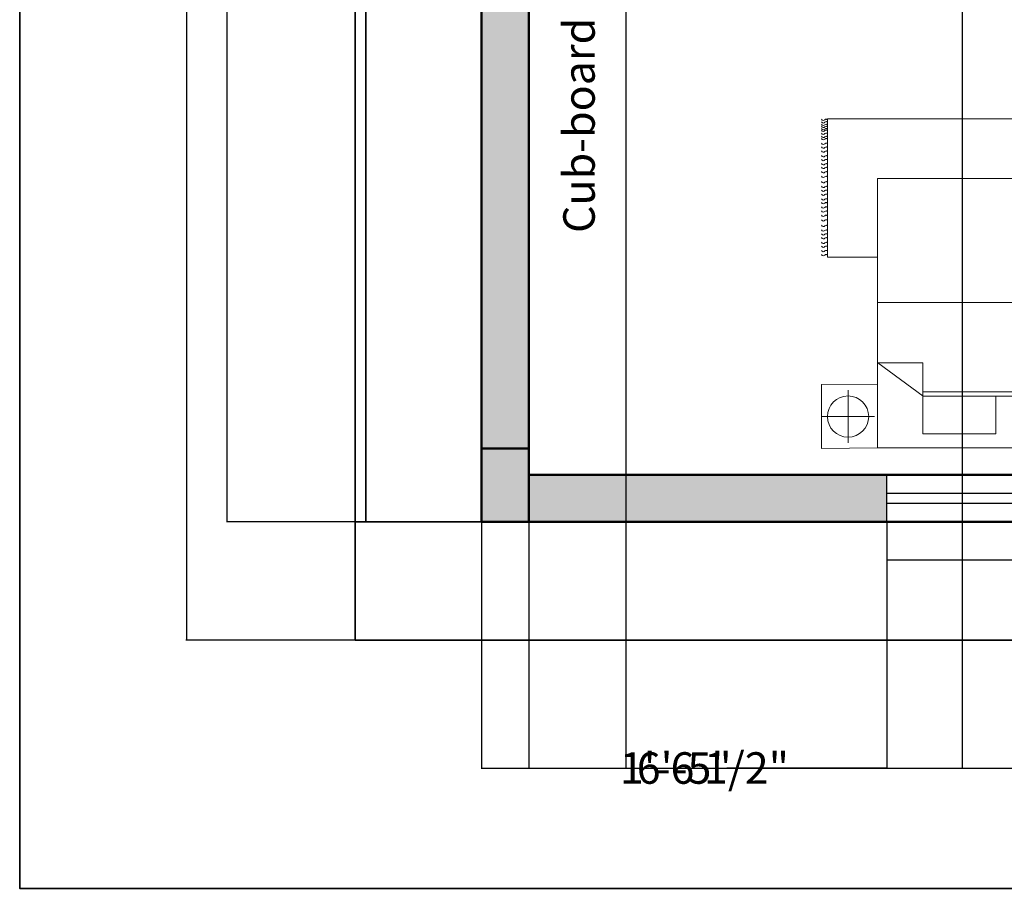
# Model space of a CAD drawing. Units: inches. Extents: x 1601 to 2080, y 5000 to 5589.
# Tile 1 of 11: x 1601 to 1788, y 5000 to 5165. Entities that reach past the tile are written whole.
import ezdxf

# ---------------------------------------------------------------- set-up
doc = ezdxf.new("R2010")
doc.units = ezdxf.units.IN
doc.header["$MEASUREMENT"] = 0
for name, color, linetype, lineweight in [('A-ANNO-DIMS', 2, 'Continuous', 18), ('A-ANNO-TEXT', 7, 'Continuous', 25), ('A-ANNO-TTLB', 7, 'Continuous', 35), ('A-COLS', 7, 'Continuous', 50), ('A-COLS-PATT', 18, 'Continuous', 13), ('A-FLOR-CASE', 8, 'Continuous', 25), ('A-FURN', 8, 'Continuous', 18), ('A-GLAZ', 4, 'Continuous', 25), ('A-WALL', 7, 'Continuous', 50), ('A-WALL-PATT', 241, 'Continuous', 13), ('C-PROP', 7, 'Continuous', 35)]:
    doc.layers.add(name, color=color, linetype=linetype, lineweight=lineweight)
doc.styles.get("Standard").update_dxf_attribs({"font": 'arial.ttf'})
doc.dimstyles.get("Standard").update_dxf_attribs({"dimtxt": 6, "dimasz": 0.18, "dimexe": 0.18, "dimexo": 0.0625, "dimgap": 0.09, "dimtad": 0, "dimtih": 1, "dimtoh": 1, "dimdec": 1, "dimzin": 0, "dimdsep": 46, "dimlunit": 3, "dimtxsty": 'Standard', "dimcen": 0.09, "dimadec": 0, "dimazin": 0, "dimtfac": 1, "dimtdec": 1, "dimtofl": 0, "dimtmove": 0, "dimatfit": 3, "dimfxl": 1, "dimtolj": 1, "dimtzin": 0, "dimarcsym": 0})

# ---------------------------------------------------------------- blocks, each defined once
blk = doc.blocks.new('*D4')
at = {"layer": 'A-ANNO-DIMS', "color": 0, "lineweight": -2, "transparency": 16777216}
for p, q in [((1664.35, 5509.2), (1632.18, 5509.2)), ((1632.36, 5509.02), (1632.36, 5281.35)), ((1632.36, 5047.39), (1632.36, 5275.05)), ((1664.35, 5047.21), (1632.18, 5047.21))]:
    blk.add_line(p, q, dxfattribs=at)
at = {"layer": 'A-ANNO-DIMS', "color": 0, "transparency": 16777216}
for points in [[(1632.33, 5509.02), (1632.39, 5509.02), (1632.36, 5509.2)], [(1632.33, 5047.39), (1632.39, 5047.39), (1632.36, 5047.21)]]:
    blk.add_solid(points, dxfattribs=at)
at = {"layer": 'Defpoints', "color": 0, "transparency": 16777216}
for p in [(1664.41, 5509.2), (1632.36, 5047.21), (1664.41, 5047.21)]:
    blk.add_point(p, dxfattribs=at)
at = {"layer": 'A-ANNO-DIMS', "color": 0, "transparency": 16777216, "insert": (1632.36, 5278.2), "char_height": 6, "attachment_point": 5}
blk.add_mtext("\\A1;40'", dxfattribs=at)
blk = doc.blocks.new('BED-DOUBLE-ENSEMBLE')
for p, q in [((5.6, 61.61), (5.6, 51.56)), ((63.65, 61.72), (63.65, 51.66)), ((10.63, 56.59), (0.57, 56.59)), ((68.68, 56.69), (58.62, 56.69)), ((49.39, 52.82), (10.63, 52.82)), ((49.39, 52.82), (58, 46.47)), ((49.44, 52.82), (49.44, 46.47)), ((49.44, 52), (10.63, 52)), ((49.44, 46.47), (58, 46.47)), ((58.05, 34.96), (10.63, 34.96)), ((4.35, 0), (4.35, 26.37)), ((4.35, 26.37), (10.65, 26.37)), ((58.05, 26.37), (67.59, 26.37)), ((67.59, 26.37), (67.59, 0)), ((67.59, 0), (4.35, 0))]:
    blk.add_line(p, q)
for points in [[(0, 50.39), (10.63, 50.5), (10.63, 62.68), (0, 62.58)], [(58.05, 62.68), (58.05, 11.36), (10.63, 11.36), (10.63, 62.68)], [(58.05, 50.5), (68.68, 50.6), (68.68, 62.78), (58.05, 62.68)], [(29.88, 59.98), (29.88, 52.82), (15.98, 52.82), (15.98, 59.98)], [(49.44, 59.98), (49.44, 52.82), (35.55, 52.82), (35.55, 59.98)]]:
    blk.add_lwpolyline(points, close=True)
for centre in [(5.6, 56.59), (63.65, 56.69)]:
    blk.add_circle(centre, 3.92)
for points, knots in [([(3.23, 25.83), (3.32, 25.96), (3.52, 26.2), (3.86, 25.96), (4.14, 25.78), (4.29, 25.89), (4.35, 25.94)], [0, 0, 0, 0, 0.400747, 0.791423, 1.067667, 1.29709, 1.29709, 1.29709, 1.29709]), ([(3.23, 25.06), (3.32, 25.18), (3.52, 25.42), (3.86, 25.18), (4.14, 25), (4.29, 25.11), (4.35, 25.16)], [0, 0, 0, 0, 0.400747, 0.791423, 1.067667, 1.29709, 1.29709, 1.29709, 1.29709]), ([(3.23, 24.24), (3.32, 24.36), (3.52, 24.6), (3.86, 24.36), (4.14, 24.19), (4.29, 24.3), (4.35, 24.34)], [0, 0, 0, 0, 0.400747, 0.791423, 1.067667, 1.29709, 1.29709, 1.29709, 1.29709]), ([(68.71, 25.83), (68.61, 25.96), (68.42, 26.2), (68.08, 25.96), (67.8, 25.78), (67.65, 25.89), (67.58, 25.94)], [0, 0, 0, 0, 0.400747, 0.791423, 1.067667, 1.29709, 1.29709, 1.29709, 1.29709]), ([(68.71, 25.06), (68.61, 25.18), (68.42, 25.42), (68.08, 25.18), (67.8, 25), (67.65, 25.11), (67.58, 25.16)], [0, 0, 0, 0, 0.400747, 0.791423, 1.067667, 1.29709, 1.29709, 1.29709, 1.29709]), ([(68.71, 24.24), (68.61, 24.36), (68.42, 24.6), (68.08, 24.36), (67.8, 24.19), (67.65, 24.3), (67.58, 24.34)], [0, 0, 0, 0, 0.400747, 0.791423, 1.067667, 1.29709, 1.29709, 1.29709, 1.29709]), ([(3.23, 23.51), (3.32, 23.63), (3.52, 23.87), (3.86, 23.63), (4.14, 23.46), (4.29, 23.57), (4.35, 23.62)], [0, 0, 0, 0, 0.400747, 0.791423, 1.067667, 1.29709, 1.29709, 1.29709, 1.29709]), ([(3.23, 22.63), (3.32, 22.75), (3.52, 22.99), (3.86, 22.75), (4.14, 22.58), (4.29, 22.68), (4.35, 22.73)], [0, 0, 0, 0, 0.400747, 0.791423, 1.067667, 1.29709, 1.29709, 1.29709, 1.29709]), ([(68.71, 23.51), (68.61, 23.63), (68.42, 23.87), (68.08, 23.63), (67.8, 23.46), (67.65, 23.57), (67.58, 23.62)], [0, 0, 0, 0, 0.400747, 0.791423, 1.067667, 1.29709, 1.29709, 1.29709, 1.29709]), ([(68.71, 22.63), (68.61, 22.75), (68.42, 22.99), (68.08, 22.75), (67.8, 22.58), (67.65, 22.68), (67.58, 22.73)], [0, 0, 0, 0, 0.400747, 0.791423, 1.067667, 1.29709, 1.29709, 1.29709, 1.29709]), ([(3.23, 21.88), (3.32, 22), (3.52, 22.24), (3.86, 22), (4.14, 21.83), (4.29, 21.93), (4.35, 21.98)], [0, 0, 0, 0, 0.400747, 0.791423, 1.067667, 1.29709, 1.29709, 1.29709, 1.29709]), ([(3.23, 21.15), (3.32, 21.27), (3.52, 21.51), (3.86, 21.27), (4.14, 21.1), (4.29, 21.2), (4.35, 21.25)], [0, 0, 0, 0, 0.400747, 0.791423, 1.067667, 1.29709, 1.29709, 1.29709, 1.29709]), ([(68.71, 21.88), (68.61, 22), (68.42, 22.24), (68.08, 22), (67.8, 21.83), (67.65, 21.93), (67.58, 21.98)], [0, 0, 0, 0, 0.400747, 0.791423, 1.067667, 1.29709, 1.29709, 1.29709, 1.29709]), ([(68.71, 21.15), (68.61, 21.27), (68.42, 21.51), (68.08, 21.27), (67.8, 21.1), (67.65, 21.2), (67.58, 21.25)], [0, 0, 0, 0, 0.400747, 0.791423, 1.067667, 1.29709, 1.29709, 1.29709, 1.29709]), ([(3.23, 20.27), (3.32, 20.39), (3.52, 20.63), (3.86, 20.39), (4.14, 20.22), (4.29, 20.32), (4.35, 20.37)], [0, 0, 0, 0, 0.400747, 0.791423, 1.067667, 1.29709, 1.29709, 1.29709, 1.29709]), ([(3.23, 19.23), (3.32, 19.35), (3.52, 19.59), (3.86, 19.35), (4.14, 19.18), (4.29, 19.29), (4.35, 19.33)], [0, 0, 0, 0, 0.400747, 0.791423, 1.067667, 1.29709, 1.29709, 1.29709, 1.29709]), ([(68.71, 20.27), (68.61, 20.39), (68.42, 20.63), (68.08, 20.39), (67.8, 20.22), (67.65, 20.32), (67.58, 20.37)], [0, 0, 0, 0, 0.400747, 0.791423, 1.067667, 1.29709, 1.29709, 1.29709, 1.29709]), ([(68.71, 19.23), (68.61, 19.35), (68.42, 19.59), (68.08, 19.35), (67.8, 19.18), (67.65, 19.29), (67.58, 19.33)], [0, 0, 0, 0, 0.400747, 0.791423, 1.067667, 1.29709, 1.29709, 1.29709, 1.29709]), ([(3.23, 18.35), (3.32, 18.47), (3.52, 18.71), (3.86, 18.47), (4.14, 18.3), (4.29, 18.4), (4.35, 18.45)], [0, 0, 0, 0, 0.400747, 0.791423, 1.067667, 1.29709, 1.29709, 1.29709, 1.29709]), ([(3.23, 17.53), (3.32, 17.65), (3.52, 17.89), (3.86, 17.65), (4.14, 17.48), (4.29, 17.59), (4.35, 17.64)], [0, 0, 0, 0, 0.400747, 0.791423, 1.067667, 1.29709, 1.29709, 1.29709, 1.29709]), ([(3.23, 16.76), (3.32, 16.88), (3.52, 17.12), (3.86, 16.88), (4.14, 16.7), (4.29, 16.81), (4.35, 16.86)], [0, 0, 0, 0, 0.400747, 0.791423, 1.067667, 1.29709, 1.29709, 1.29709, 1.29709]), ([(68.71, 18.35), (68.61, 18.47), (68.42, 18.71), (68.08, 18.47), (67.8, 18.3), (67.65, 18.4), (67.58, 18.45)], [0, 0, 0, 0, 0.400747, 0.791423, 1.067667, 1.29709, 1.29709, 1.29709, 1.29709]), ([(68.71, 17.53), (68.61, 17.65), (68.42, 17.89), (68.08, 17.65), (67.8, 17.48), (67.65, 17.59), (67.58, 17.64)], [0, 0, 0, 0, 0.400747, 0.791423, 1.067667, 1.29709, 1.29709, 1.29709, 1.29709]), ([(68.71, 16.76), (68.61, 16.88), (68.42, 17.12), (68.08, 16.88), (67.8, 16.7), (67.65, 16.81), (67.58, 16.86)], [0, 0, 0, 0, 0.400747, 0.791423, 1.067667, 1.29709, 1.29709, 1.29709, 1.29709]), ([(3.23, 15.94), (3.32, 16.06), (3.52, 16.3), (3.86, 16.06), (4.14, 15.89), (4.29, 15.99), (4.35, 16.04)], [0, 0, 0, 0, 0.400747, 0.791423, 1.067667, 1.29709, 1.29709, 1.29709, 1.29709]), ([(3.23, 15.21), (3.32, 15.33), (3.52, 15.57), (3.86, 15.33), (4.14, 15.16), (4.29, 15.27), (4.35, 15.31)], [0, 0, 0, 0, 0.400747, 0.791423, 1.067667, 1.29709, 1.29709, 1.29709, 1.29709]), ([(68.71, 15.94), (68.61, 16.06), (68.42, 16.3), (68.08, 16.06), (67.8, 15.89), (67.65, 15.99), (67.58, 16.04)], [0, 0, 0, 0, 0.400747, 0.791423, 1.067667, 1.29709, 1.29709, 1.29709, 1.29709]), ([(68.71, 15.21), (68.61, 15.33), (68.42, 15.57), (68.08, 15.33), (67.8, 15.16), (67.65, 15.27), (67.58, 15.31)], [0, 0, 0, 0, 0.400747, 0.791423, 1.067667, 1.29709, 1.29709, 1.29709, 1.29709]), ([(3.23, 14.33), (3.32, 14.45), (3.52, 14.69), (3.86, 14.45), (4.14, 14.28), (4.29, 14.38), (4.35, 14.43)], [0, 0, 0, 0, 0.400747, 0.791423, 1.067667, 1.29709, 1.29709, 1.29709, 1.29709]), ([(3.23, 13.58), (3.32, 13.7), (3.52, 13.94), (3.86, 13.7), (4.14, 13.53), (4.29, 13.63), (4.35, 13.68)], [0, 0, 0, 0, 0.400747, 0.791423, 1.067667, 1.29709, 1.29709, 1.29709, 1.29709]), ([(3.23, 12.85), (3.32, 12.97), (3.52, 13.21), (3.86, 12.97), (4.14, 12.8), (4.29, 12.9), (4.35, 12.95)], [0, 0, 0, 0, 0.400747, 0.791423, 1.067667, 1.29709, 1.29709, 1.29709, 1.29709]), ([(68.71, 14.33), (68.61, 14.45), (68.42, 14.69), (68.08, 14.45), (67.8, 14.28), (67.65, 14.38), (67.58, 14.43)], [0, 0, 0, 0, 0.400747, 0.791423, 1.067667, 1.29709, 1.29709, 1.29709, 1.29709]), ([(68.71, 13.58), (68.61, 13.7), (68.42, 13.94), (68.08, 13.7), (67.8, 13.53), (67.65, 13.63), (67.58, 13.68)], [0, 0, 0, 0, 0.400747, 0.791423, 1.067667, 1.29709, 1.29709, 1.29709, 1.29709]), ([(68.71, 12.85), (68.61, 12.97), (68.42, 13.21), (68.08, 12.97), (67.8, 12.8), (67.65, 12.9), (67.58, 12.95)], [0, 0, 0, 0, 0.400747, 0.791423, 1.067667, 1.29709, 1.29709, 1.29709, 1.29709]), ([(3.23, 11.97), (3.32, 12.09), (3.52, 12.33), (3.86, 12.09), (4.14, 11.92), (4.29, 12.02), (4.35, 12.07)], [0, 0, 0, 0, 0.400747, 0.791423, 1.067667, 1.29709, 1.29709, 1.29709, 1.29709]), ([(68.71, 11.97), (68.61, 12.09), (68.42, 12.33), (68.08, 12.09), (67.8, 11.92), (67.65, 12.02), (67.58, 12.07)], [0, 0, 0, 0, 0.400747, 0.791423, 1.067667, 1.29709, 1.29709, 1.29709, 1.29709]), ([(3.23, 10.93), (3.32, 11.05), (3.52, 11.29), (3.86, 11.05), (4.14, 10.88), (4.29, 10.99), (4.35, 11.03)], [0, 0, 0, 0, 0.400747, 0.791423, 1.067667, 1.29709, 1.29709, 1.29709, 1.29709]), ([(3.23, 10.05), (3.32, 10.17), (3.52, 10.41), (3.86, 10.17), (4.14, 10), (4.29, 10.1), (4.35, 10.15)], [0, 0, 0, 0, 0.400747, 0.791423, 1.067667, 1.29709, 1.29709, 1.29709, 1.29709]), ([(3.23, 9.23), (3.32, 9.35), (3.52, 9.59), (3.86, 9.35), (4.14, 9.18), (4.29, 9.29), (4.35, 9.34)], [0, 0, 0, 0, 0.400747, 0.791423, 1.067667, 1.29709, 1.29709, 1.29709, 1.29709]), ([(68.71, 10.93), (68.61, 11.05), (68.42, 11.29), (68.08, 11.05), (67.8, 10.88), (67.65, 10.99), (67.58, 11.03)], [0, 0, 0, 0, 0.400747, 0.791423, 1.067667, 1.29709, 1.29709, 1.29709, 1.29709]), ([(68.71, 10.05), (68.61, 10.17), (68.42, 10.41), (68.08, 10.17), (67.8, 10), (67.65, 10.1), (67.58, 10.15)], [0, 0, 0, 0, 0.400747, 0.791423, 1.067667, 1.29709, 1.29709, 1.29709, 1.29709]), ([(68.71, 9.23), (68.61, 9.35), (68.42, 9.59), (68.08, 9.35), (67.8, 9.18), (67.65, 9.29), (67.58, 9.34)], [0, 0, 0, 0, 0.400747, 0.791423, 1.067667, 1.29709, 1.29709, 1.29709, 1.29709]), ([(3.23, 8.54), (3.32, 8.66), (3.52, 8.9), (3.86, 8.66), (4.14, 8.49), (4.29, 8.6), (4.35, 8.65)], [0, 0, 0, 0, 0.400747, 0.791423, 1.067667, 1.29709, 1.29709, 1.29709, 1.29709]), ([(3.23, 7.73), (3.32, 7.85), (3.52, 8.09), (3.86, 7.85), (4.14, 7.67), (4.29, 7.78), (4.35, 7.83)], [0, 0, 0, 0, 0.400747, 0.791423, 1.067667, 1.29709, 1.29709, 1.29709, 1.29709]), ([(68.71, 8.54), (68.61, 8.66), (68.42, 8.9), (68.08, 8.66), (67.8, 8.49), (67.65, 8.6), (67.58, 8.65)], [0, 0, 0, 0, 0.400747, 0.791423, 1.067667, 1.29709, 1.29709, 1.29709, 1.29709]), ([(68.71, 7.73), (68.61, 7.85), (68.42, 8.09), (68.08, 7.85), (67.8, 7.67), (67.65, 7.78), (67.58, 7.83)], [0, 0, 0, 0, 0.400747, 0.791423, 1.067667, 1.29709, 1.29709, 1.29709, 1.29709]), ([(3.23, 7), (3.32, 7.12), (3.52, 7.36), (3.86, 7.12), (4.14, 6.95), (4.29, 7.05), (4.35, 7.1)], [0, 0, 0, 0, 0.400747, 0.791423, 1.067667, 1.29709, 1.29709, 1.29709, 1.29709]), ([(3.23, 6.12), (3.32, 6.24), (3.52, 6.48), (3.86, 6.24), (4.14, 6.06), (4.29, 6.17), (4.35, 6.22)], [0, 0, 0, 0, 0.400747, 0.791423, 1.067667, 1.29709, 1.29709, 1.29709, 1.29709]), ([(3.23, 5.36), (3.32, 5.49), (3.52, 5.72), (3.86, 5.49), (4.14, 5.31), (4.29, 5.42), (4.35, 5.47)], [0, 0, 0, 0, 0.400747, 0.791423, 1.067667, 1.29709, 1.29709, 1.29709, 1.29709]), ([(68.71, 7), (68.61, 7.12), (68.42, 7.36), (68.08, 7.12), (67.8, 6.95), (67.65, 7.05), (67.58, 7.1)], [0, 0, 0, 0, 0.400747, 0.791423, 1.067667, 1.29709, 1.29709, 1.29709, 1.29709]), ([(68.71, 6.12), (68.61, 6.24), (68.42, 6.48), (68.08, 6.24), (67.8, 6.06), (67.65, 6.17), (67.58, 6.22)], [0, 0, 0, 0, 0.400747, 0.791423, 1.067667, 1.29709, 1.29709, 1.29709, 1.29709]), ([(68.71, 5.36), (68.61, 5.49), (68.42, 5.72), (68.08, 5.49), (67.8, 5.31), (67.65, 5.42), (67.58, 5.47)], [0, 0, 0, 0, 0.400747, 0.791423, 1.067667, 1.29709, 1.29709, 1.29709, 1.29709]), ([(3.23, 4.64), (3.32, 4.76), (3.52, 5), (3.86, 4.76), (4.14, 4.58), (4.29, 4.69), (4.35, 4.74)], [0, 0, 0, 0, 0.400747, 0.791423, 1.067667, 1.29709, 1.29709, 1.29709, 1.29709]), ([(3.23, 3.75), (3.32, 3.88), (3.52, 4.11), (3.86, 3.88), (4.14, 3.7), (4.29, 3.81), (4.35, 3.86)], [0, 0, 0, 0, 0.400747, 0.791423, 1.067667, 1.29709, 1.29709, 1.29709, 1.29709]), ([(68.71, 4.64), (68.61, 4.76), (68.42, 5), (68.08, 4.76), (67.8, 4.59), (67.66, 4.69), (67.59, 4.73)], [0, 0, 0, 0, 0.400747, 0.791423, 1.067667, 1.283686, 1.283686, 1.283686, 1.283686]), ([(68.71, 3.75), (68.61, 3.88), (68.42, 4.11), (68.08, 3.88), (67.8, 3.7), (67.66, 3.8), (67.59, 3.85)], [0, 0, 0, 0, 0.400747, 0.791423, 1.067667, 1.283686, 1.283686, 1.283686, 1.283686]), ([(3.23, 3.32), (3.32, 3.45), (3.51, 3.7), (3.86, 3.44), (4.14, 3.27), (4.29, 3.38), (4.35, 3.43)], [0, 0, 0, 0, 0.407265, 0.802015, 1.07826, 1.307683, 1.307683, 1.307683, 1.307683]), ([(3.23, 2.76), (3.32, 2.88), (3.52, 3.12), (3.86, 2.88), (4.14, 2.71), (4.29, 2.81), (4.35, 2.86)], [0, 0, 0, 0, 0.400747, 0.791423, 1.067667, 1.29709, 1.29709, 1.29709, 1.29709]), ([(3.23, 2.18), (3.32, 2.31), (3.52, 2.54), (3.86, 2.31), (4.14, 2.13), (4.29, 2.24), (4.35, 2.29)], [0, 0, 0, 0, 0.400747, 0.791423, 1.067667, 1.29709, 1.29709, 1.29709, 1.29709]), ([(3.23, 1.88), (3.32, 2), (3.52, 2.24), (3.86, 2), (4.14, 1.82), (4.29, 1.93), (4.35, 1.98)], [0, 0, 0, 0, 0.400747, 0.791423, 1.067667, 1.29709, 1.29709, 1.29709, 1.29709]), ([(68.71, 3.32), (68.61, 3.45), (68.42, 3.69), (68.08, 3.45), (67.8, 3.27), (67.66, 3.38), (67.59, 3.42)], [0, 0, 0, 0, 0.402903, 0.794912, 1.071156, 1.287177, 1.287177, 1.287177, 1.287177]), ([(68.71, 2.73), (68.61, 2.85), (68.42, 3.09), (68.08, 2.85), (67.8, 2.68), (67.66, 2.78), (67.59, 2.82)], [0, 0, 0, 0, 0.400747, 0.791423, 1.067667, 1.283686, 1.283686, 1.283686, 1.283686]), ([(68.71, 2.16), (68.61, 2.28), (68.42, 2.52), (68.08, 2.28), (67.8, 2.11), (67.66, 2.21), (67.59, 2.25)], [0, 0, 0, 0, 0.400747, 0.791423, 1.067667, 1.283686, 1.283686, 1.283686, 1.283686]), ([(68.71, 1.85), (68.61, 1.97), (68.42, 2.21), (68.08, 1.97), (67.8, 1.8), (67.66, 1.9), (67.59, 1.94)], [0, 0, 0, 0, 0.400747, 0.791423, 1.067667, 1.283686, 1.283686, 1.283686, 1.283686]), ([(3.23, 1.46), (3.32, 1.58), (3.52, 1.82), (3.86, 1.58), (4.14, 1.4), (4.29, 1.51), (4.35, 1.56)], [0, 0, 0, 0, 0.400747, 0.791423, 1.067667, 1.29709, 1.29709, 1.29709, 1.29709]), ([(3.23, 1.06), (3.32, 1.18), (3.52, 1.42), (3.86, 1.18), (4.14, 1.01), (4.29, 1.11), (4.35, 1.16)], [0, 0, 0, 0, 0.400747, 0.791423, 1.067667, 1.29709, 1.29709, 1.29709, 1.29709]), ([(3.23, 0.57), (3.32, 0.7), (3.52, 0.93), (3.86, 0.7), (4.14, 0.52), (4.29, 0.63), (4.35, 0.68)], [0, 0, 0, 0, 0.400747, 0.791423, 1.067667, 1.29709, 1.29709, 1.29709, 1.29709]), ([(3.23, 0.07), (3.32, 0.19), (3.52, 0.43), (3.86, 0.19), (4.14, 0.02), (4.29, 0.13), (4.35, 0.18)], [0, 0, 0, 0, 0.400747, 0.791423, 1.067667, 1.29709, 1.29709, 1.29709, 1.29709]), ([(68.71, 1.43), (68.61, 1.55), (68.42, 1.79), (68.08, 1.55), (67.8, 1.38), (67.65, 1.48), (67.58, 1.53)], [0, 0, 0, 0, 0.400747, 0.791423, 1.067667, 1.29709, 1.29709, 1.29709, 1.29709]), ([(68.71, 1.03), (68.61, 1.15), (68.42, 1.39), (68.08, 1.15), (67.8, 0.98), (67.65, 1.09), (67.58, 1.13)], [0, 0, 0, 0, 0.400747, 0.791423, 1.067667, 1.29709, 1.29709, 1.29709, 1.29709]), ([(68.71, 0.55), (68.61, 0.67), (68.42, 0.91), (68.08, 0.67), (67.8, 0.49), (67.65, 0.6), (67.58, 0.65)], [0, 0, 0, 0, 0.400747, 0.791423, 1.067667, 1.29709, 1.29709, 1.29709, 1.29709]), ([(68.71, 0.07), (68.61, 0.19), (68.42, 0.43), (68.08, 0.19), (67.8, 0.02), (67.65, 0.13), (67.58, 0.18)], [0, 0, 0, 0, 0.400747, 0.791423, 1.067667, 1.29709, 1.29709, 1.29709, 1.29709])]:
    blk.add_open_spline(points, degree=3, knots=knots)
blk = doc.blocks.new('WINDOW-48IN')
for p, q in [((0, 0), (0, 9)), ((0, 9), (48, 9)), ((48, 9), (48, 0)), ((0, 5.5), (48, 5.5)), ((48, 3.5), (0, 3.5)), ((48, 0), (0, 0))]:
    blk.add_line(p, q)
blk = doc.blocks.new('*D15')
at = {"layer": 'A-ANNO-DIMS', "color": 0, "lineweight": -2, "transparency": 16777216}
for p, q in [((1765.58, 5069.63), (1765.58, 5062.32)), ((1813.58, 5069.63), (1813.58, 5062.32)), ((1765.76, 5062.5), (1813.4, 5062.5)), ((1813.58, 5062.5), (1813.76, 5062.5))]:
    blk.add_line(p, q, dxfattribs=at)
at = {"layer": 'A-ANNO-DIMS', "color": 0, "transparency": 16777216}
for points in [[(1765.76, 5062.53), (1765.76, 5062.47), (1765.58, 5062.5)], [(1813.4, 5062.53), (1813.4, 5062.47), (1813.58, 5062.5)]]:
    blk.add_solid(points, dxfattribs=at)
at = {"layer": 'Defpoints', "color": 0, "transparency": 16777216}
for p in [(1765.58, 5069.7), (1813.58, 5069.7), (1813.58, 5062.5)]:
    blk.add_point(p, dxfattribs=at)
at = {"layer": 'A-ANNO-DIMS', "color": 0, "transparency": 16777216, "insert": (1851.82, 5062.5), "char_height": 6, "attachment_point": 5}
blk.add_mtext('\\A1;WINDOW 4\'-0" TYP.', dxfattribs=at)
blk = doc.blocks.new('*D37')
at = {"layer": 'A-ANNO-DIMS', "color": 0, "lineweight": -2, "transparency": 16777216}
for p, q in [((1688.41, 5069.63), (1688.41, 5022.68)), ((1962.91, 5069.63), (1962.91, 5022.68)), ((1688.59, 5022.86), (1805.89, 5022.86)), ((1962.73, 5022.86), (1845.43, 5022.86))]:
    blk.add_line(p, q, dxfattribs=at)
at = {"layer": 'A-ANNO-DIMS', "color": 0, "transparency": 16777216}
for points in [[(1688.59, 5022.89), (1688.59, 5022.83), (1688.41, 5022.86)], [(1962.73, 5022.89), (1962.73, 5022.83), (1962.91, 5022.86)]]:
    blk.add_solid(points, dxfattribs=at)
at = {"layer": 'Defpoints', "color": 0, "transparency": 16777216}
for p in [(1688.41, 5069.7), (1962.91, 5069.7), (1962.91, 5022.86)]:
    blk.add_point(p, dxfattribs=at)
at = {"layer": 'A-ANNO-DIMS', "color": 0, "transparency": 16777216, "insert": (1825.66, 5022.86), "char_height": 6, "attachment_point": 5}
blk.add_mtext('\\A1;22\'-10 1/2"', dxfattribs=at)
blk = doc.blocks.new('*D38')
at = {"layer": 'A-ANNO-DIMS', "color": 0, "lineweight": -2, "transparency": 16777216}
for p, q in [((1688.35, 5431.2), (1639.88, 5431.2)), ((1640.06, 5431.02), (1640.06, 5253.64)), ((1640.06, 5069.88), (1640.06, 5247.25)), ((1688.35, 5069.7), (1639.88, 5069.7))]:
    blk.add_line(p, q, dxfattribs=at)
at = {"layer": 'A-ANNO-DIMS', "color": 0, "transparency": 16777216}
for points in [[(1640.03, 5431.02), (1640.09, 5431.02), (1640.06, 5431.2)], [(1640.03, 5069.88), (1640.09, 5069.88), (1640.06, 5069.7)]]:
    blk.add_solid(points, dxfattribs=at)
at = {"layer": 'Defpoints', "color": 0, "transparency": 16777216}
for p in [(1640.06, 5431.2), (1688.41, 5431.2), (1688.41, 5069.7)]:
    blk.add_point(p, dxfattribs=at)
at = {"layer": 'A-ANNO-DIMS', "color": 0, "transparency": 16777216, "insert": (1640.06, 5250.45), "char_height": 6, "attachment_point": 5}
blk.add_mtext('\\A1;30\'-1 1/2"', dxfattribs=at)
blk = doc.blocks.new('*D43')
at = {"layer": 'A-ANNO-DIMS', "color": 0, "lineweight": -2, "transparency": 16777216}
for p, q in [((1697.41, 5078.63), (1697.41, 5022.68)), ((1715.89, 5078.63), (1715.89, 5022.68)), ((1697.59, 5022.86), (1715.71, 5022.86)), ((1715.89, 5022.86), (1716.07, 5022.86))]:
    blk.add_line(p, q, dxfattribs=at)
at = {"layer": 'A-ANNO-DIMS', "color": 0, "transparency": 16777216}
for points in [[(1697.59, 5022.89), (1697.59, 5022.83), (1697.41, 5022.86)], [(1715.71, 5022.89), (1715.71, 5022.83), (1715.89, 5022.86)]]:
    blk.add_solid(points, dxfattribs=at)
at = {"layer": 'Defpoints', "color": 0, "transparency": 16777216}
for p in [(1697.41, 5078.7), (1715.89, 5078.7), (1715.89, 5022.86)]:
    blk.add_point(p, dxfattribs=at)
at = {"layer": 'A-ANNO-DIMS', "color": 0, "transparency": 16777216, "insert": (1730.84, 5022.86), "char_height": 6, "attachment_point": 5}
blk.add_mtext('\\A1;1\'-6 1/2"', dxfattribs=at)
blk = doc.blocks.new('*D46')
at = {"layer": 'A-ANNO-DIMS', "color": 0, "lineweight": -2, "transparency": 16777216}
for p, q in [((1688.41, 5069.63), (1688.41, 5022.68)), ((1765.58, 5069.63), (1765.58, 5022.68)), ((1688.59, 5022.86), (1718.91, 5022.86)), ((1765.4, 5022.86), (1735.08, 5022.86))]:
    blk.add_line(p, q, dxfattribs=at)
at = {"layer": 'A-ANNO-DIMS', "color": 0, "transparency": 16777216}
for points in [[(1688.59, 5022.89), (1688.59, 5022.83), (1688.41, 5022.86)], [(1765.4, 5022.89), (1765.4, 5022.83), (1765.58, 5022.86)]]:
    blk.add_solid(points, dxfattribs=at)
at = {"layer": 'Defpoints', "color": 0, "transparency": 16777216}
for p in [(1688.41, 5069.7), (1765.58, 5069.7), (1765.58, 5022.86)]:
    blk.add_point(p, dxfattribs=at)
at = {"layer": 'A-ANNO-DIMS', "color": 0, "transparency": 16777216, "insert": (1727, 5022.86), "char_height": 6, "attachment_point": 5}
blk.add_mtext('\\A1;6\'-5"', dxfattribs=at)
blk = doc.blocks.new('*D58')
at = {"layer": 'A-ANNO-DIMS', "color": 0, "lineweight": -2, "transparency": 16777216}
for p, q in [((1779.91, 5209.13), (1779.91, 5022.68)), ((1824.91, 5209.13), (1824.91, 5022.68)), ((1780.09, 5022.86), (1794.35, 5022.86)), ((1824.73, 5022.86), (1810.47, 5022.86))]:
    blk.add_line(p, q, dxfattribs=at)
at = {"layer": 'A-ANNO-DIMS', "color": 0, "transparency": 16777216}
for points in [[(1780.09, 5022.89), (1780.09, 5022.83), (1779.91, 5022.86)], [(1824.73, 5022.89), (1824.73, 5022.83), (1824.91, 5022.86)]]:
    blk.add_solid(points, dxfattribs=at)
at = {"layer": 'Defpoints', "color": 0, "transparency": 16777216}
for p in [(1779.91, 5209.2), (1824.91, 5209.2), (1824.91, 5022.86)]:
    blk.add_point(p, dxfattribs=at)
at = {"layer": 'A-ANNO-DIMS', "color": 0, "transparency": 16777216, "insert": (1802.41, 5022.86), "char_height": 6, "attachment_point": 5}
blk.add_mtext('\\A1;3\'-9"', dxfattribs=at)

msp = doc.modelspace()

# ---------------------------------------------------------------- hatches: boundary and pattern name
at = {"layer": 'A-COLS-PATT'}
h = msp.add_hatch(color=256, dxfattribs=at)
h.dxf.hatch_style = 1
h.paths.add_polyline_path([(1702.41, 5431.2), (1688.41, 5431.2), (1688.41, 5422.2), (1702.41, 5422.2)])
h.paths.add_polyline_path([(1836.17, 5431.2), (1822.17, 5431.2), (1822.17, 5422.2), (1836.17, 5422.2)])
h.paths.add_polyline_path([(1962.91, 5431.2), (1948.91, 5431.2), (1948.91, 5422.2), (1962.91, 5422.2)])
h.paths.add_polyline_path([(1697.41, 5314.2), (1688.41, 5314.2), (1688.41, 5300.2), (1697.41, 5300.2)])
h.paths.add_polyline_path([(1833.91, 5314.2), (1824.91, 5314.2), (1824.91, 5300.2), (1833.91, 5300.2)])
h.paths.add_polyline_path([(1962.91, 5314.2), (1953.91, 5314.2), (1953.91, 5300.2), (1962.91, 5300.2)])
h.paths.add_polyline_path([(1697.41, 5209.2), (1688.41, 5209.2), (1688.41, 5195.2), (1697.41, 5195.2)])
h.paths.add_polyline_path([(1833.91, 5209.2), (1824.91, 5209.2), (1824.91, 5195.2), (1833.91, 5195.2)])
h.paths.add_polyline_path([(1962.91, 5209.2), (1953.91, 5209.2), (1953.91, 5195.2), (1962.91, 5195.2)])
h.paths.add_polyline_path([(1697.41, 5083.7), (1688.41, 5083.7), (1688.41, 5069.7), (1697.41, 5069.7)])
h.paths.add_polyline_path([(1833.91, 5078.7), (1819.91, 5078.7), (1819.91, 5069.7), (1833.91, 5069.7)])
h.paths.add_polyline_path([(1962.91, 5078.7), (1948.91, 5078.7), (1948.91, 5069.7), (1962.91, 5069.7)])
at = {"layer": 'A-WALL-PATT'}
h = msp.add_hatch(color=256, dxfattribs=at)
h.dxf.hatch_style = 1
h.paths.add_polyline_path([(1763.95, 5431.2), (1702.41, 5431.2), (1702.41, 5422.2), (1763.95, 5422.2)])
h.paths.add_polyline_path([(1697.41, 5422.2), (1688.41, 5422.2), (1688.41, 5314.2), (1697.41, 5314.2)])
h.paths.add_polyline_path([(1740.41, 5314.2), (1697.41, 5314.2), (1697.41, 5309.7), (1740.41, 5309.7)], flags=17)
h.paths.add_polyline_path([(1822.17, 5431.2), (1811.95, 5431.2), (1811.95, 5422.2), (1822.17, 5422.2)])
h.paths.add_polyline_path([(1845.52, 5431.2), (1836.17, 5431.2), (1836.17, 5422.2), (1845.52, 5422.2)])
h.paths.add_polyline_path([(1910.91, 5431.2), (1881.52, 5431.2), (1881.52, 5422.2), (1910.91, 5422.2)])
h.paths.add_polyline_path([(1948.91, 5431.2), (1945.91, 5431.2), (1942.91, 5431.2), (1942.91, 5422.2), (1948.91, 5422.2)])
h.paths.add_polyline_path([(1962.91, 5422.2), (1953.91, 5422.2), (1953.91, 5416.29), (1962.91, 5416.29)])
h.paths.add_polyline_path([(1962.91, 5384.29), (1953.91, 5384.29), (1953.91, 5381.29), (1962.91, 5381.29)])
h.paths.add_polyline_path([(1962.91, 5333.29), (1953.91, 5333.29), (1953.91, 5314.2), (1962.91, 5314.2)])
h.paths.add_polyline_path([(1962.91, 5300.2), (1953.91, 5300.2), (1953.91, 5236.2), (1875.91, 5236.2), (1875.91, 5230.7), (1881.91, 5230.7), (1881.91, 5231.7), (1953.91, 5231.7), (1953.91, 5219.2), (1962.91, 5219.2)])
h.paths.add_polyline_path([(1962.91, 5185.2), (1953.91, 5185.2), (1953.91, 5183.7), (1881.91, 5183.7), (1881.91, 5184.7), (1875.91, 5184.7), (1875.91, 5183.7), (1875.91, 5179.2), (1953.91, 5179.2), (1953.91, 5172.6), (1962.91, 5172.6)])
h.paths.add_polyline_path([(1962.91, 5136.6), (1953.91, 5136.6), (1953.91, 5078.7), (1962.91, 5078.7)])
h.paths.add_polyline_path([(1948.91, 5078.7), (1833.91, 5078.7), (1833.91, 5069.7), (1948.91, 5069.7)])
h.paths.add_polyline_path([(1833.91, 5195.2), (1829.41, 5195.2), (1829.41, 5078.7), (1833.91, 5078.7)])
h.paths.add_polyline_path([(1819.91, 5078.7), (1813.58, 5078.7), (1813.58, 5069.7), (1819.91, 5069.7)])
h.paths.add_polyline_path([(1765.58, 5078.7), (1697.41, 5078.7), (1697.41, 5069.7), (1765.58, 5069.7)])
h.paths.add_polyline_path([(1697.41, 5195.2), (1688.41, 5195.2), (1688.41, 5083.7), (1697.41, 5083.7)])
h.paths.add_polyline_path([(1740.41, 5209.2), (1697.41, 5209.2), (1697.41, 5204.7), (1740.41, 5204.7)], flags=17)
h.paths.add_polyline_path([(1787.91, 5209.2), (1779.91, 5209.2), (1779.91, 5309.7), (1787.91, 5309.7), (1787.91, 5314.2), (1772.41, 5314.2), (1772.41, 5309.7), (1775.41, 5309.7), (1775.41, 5261.7), (1697.41, 5261.7), (1697.41, 5273.07), (1688.41, 5273.07), (1688.41, 5242.37), (1697.41, 5242.37), (1697.41, 5257.2), (1775.41, 5257.2), (1775.41, 5209.2), (1772.41, 5209.2), (1772.41, 5204.7), (1775.41, 5204.7), (1787.91, 5204.7)])
h.paths.add_polyline_path([(1697.41, 5218.37), (1688.41, 5218.37), (1688.41, 5209.2), (1697.41, 5209.2)], flags=17)
h.paths.add_polyline_path([(1833.91, 5422.2), (1829.41, 5422.2), (1829.41, 5314.2), (1833.91, 5314.2)])
h.paths.add_polyline_path([(1697.41, 5300.2), (1688.41, 5300.2), (1688.41, 5297.07), (1697.41, 5297.07)], flags=17)

# ---------------------------------------------------------------- linework, layer by layer
at = {"layer": 'A-ANNO-TTLB'}
msp.add_lwpolyline([(1600.55, 5589.45), (2079.72, 5589.45), (2079.72, 4999.95), (1600.55, 4999.95)], close=True, dxfattribs=at)
at = {"layer": 'A-COLS'}
msp.add_line((1688.41, 5083.7), (1697.41, 5083.7), dxfattribs=at)
at = {"layer": 'A-FLOR-CASE'}
msp.add_line((1715.89, 5204.7), (1715.89, 5078.7), dxfattribs=at)
at = {"layer": 'A-WALL'}
for p, q in [((1688.41, 5431.2), (1688.41, 5069.7)), ((1697.41, 5257.2), (1697.41, 5069.7)), ((1697.41, 5078.7), (1962.91, 5078.7)), ((1688.41, 5069.7), (1962.91, 5069.7))]:
    msp.add_line(p, q, dxfattribs=at)
at = {"layer": 'C-PROP'}
for p, q in [((1664.41, 5509.2), (1664.41, 5047.21)), ((1666.41, 5507.2), (1666.41, 5069.7)), ((1664.41, 5069.7), (1688.41, 5069.7)), ((1664.41, 5047.21), (2022.91, 5047.21))]:
    msp.add_line(p, q, dxfattribs=at)

# ---------------------------------------------------------------- block references
at = {"layer": 'A-FURN', "rotation": 180}
msp.add_blockref('BED-DOUBLE-ENSEMBLE', (1821.83, 5146.47), dxfattribs=at)
at = {"layer": 'A-GLAZ'}
msp.add_blockref('WINDOW-48IN', (1765.58, 5069.7), dxfattribs=at)

# ---------------------------------------------------------------- texts
at = {"layer": 'A-ANNO-TEXT', "insert": (1703.98, 5124.74), "char_height": 6, "attachment_point": 1, "rotation": 90}
msp.add_mtext_dynamic_manual_height_columns('Cub-board', width=45.9316, gutter_width=30, heights=[0], dxfattribs=at)

# ---------------------------------------------------------------- dimensions: what is measured, and where the dimension line sits
at = {"layer": 'A-ANNO-DIMS'}
dim = msp.add_linear_dim(base=(1632.36, 5047.21), p1=(1664.41, 5509.2), p2=(1664.41, 5047.21), angle=90, text="40'", dimstyle='Standard', override={"dimclrd": 0, "dimclre": 0, "dimclrt": 0}, dxfattribs=at)
dim.commit()
dim.dimension.update_dxf_attribs({"geometry": '*D4', "text_midpoint": (1632.36, 5278.2)})
dim = msp.add_linear_dim(base=(1640.06, 5431.2), p1=(1688.41, 5069.7), p2=(1688.41, 5431.2), angle=90, dimstyle='Standard', override={"dimdec": 1, "dimlfac": 1, "dimrnd": 0, "dimzin": 1, "dimdsep": 46, "dimlunit": 4, "dimfrac": 2}, dxfattribs=at)
dim.commit()
dim.dimension.update_dxf_attribs({"geometry": '*D38', "text_midpoint": (1640.06, 5250.45)})
for base, p1, p2, picture, middle in [((1824.91, 5022.86), (1779.91, 5209.2), (1824.91, 5209.2), '*D58', (1802.41, 5022.86)), ((1715.89, 5022.86), (1697.41, 5078.7), (1715.89, 5078.7), '*D43', (1730.84, 5022.86)), ((1962.91, 5022.86), (1688.41, 5069.7), (1962.91, 5069.7), '*D37', (1825.66, 5022.86)), ((1765.58, 5022.86), (1688.41, 5069.7), (1765.58, 5069.7), '*D46', (1727, 5022.86))]:
    dim = msp.add_linear_dim(base=base, p1=p1, p2=p2, dimstyle='Standard', override={"dimdec": 1, "dimlfac": 1, "dimrnd": 0, "dimzin": 1, "dimdsep": 46, "dimlunit": 4, "dimfrac": 2}, dxfattribs=at)
    dim.commit()
    dim.dimension.update_dxf_attribs({"geometry": picture, "text_midpoint": middle})
dim = msp.add_linear_dim(base=(1813.58, 5062.5), p1=(1765.58, 5069.7), p2=(1813.58, 5069.7), text='WINDOW <> TYP.', dimstyle='Standard', override={"dimdec": 1, "dimlfac": 1, "dimrnd": 0, "dimzin": 1, "dimdsep": 46, "dimlunit": 4, "dimfrac": 2}, dxfattribs=at)
dim.commit()
dim.dimension.update_dxf_attribs({"geometry": '*D15', "text_midpoint": (1851.82, 5062.5)})

doc.saveas('drawing.dxf')
